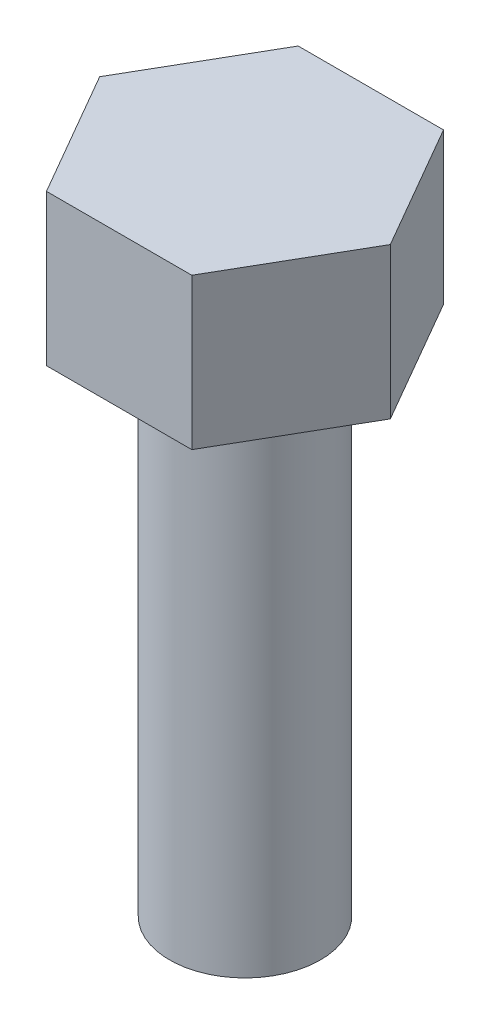
SolidWorks part; units mm, degrees
material "Plain Carbon Steel"
ref_plane "Front Plane" through (0, 0, 0) normal (0, 0, 1) x (1, 0, 0)
ref_plane "Top Plane" through (0, 0, 0) normal (0, 1, 0) x (1, 0, 0)
ref_plane "Right Plane" through (0, 0, 0) normal (1, 0, 0) x (0, 0, -1)
sketch "Hex Head Profile" plane through (0, 0, 0) normal (0, 1, 0) x (1, 0, 0)
  line L1 (2.8868, 0) -> (1.4434, 2.5)
  line L2 (1.4434, 2.5) -> (-1.4434, 2.5)
  line L3 (-1.4434, 2.5) -> (-2.8868, 0)
  line L4 (-2.8868, 0) -> (-1.4434, -2.5)
  line L5 (-1.4434, -2.5) -> (1.4434, -2.5)
  line L6 (1.4434, -2.5) -> (2.8868, 0)
  circle A0 centre (0, 0) radius 2.5 construction
  dimension "D1" = 5
extrude "Hex Head 5AF x 3" add sketch "Hex Head Profile" along normal blind 3
sketch "Shank Profile Ø3" plane through (0, 0, 0) normal (0, -1, 0) x (1, 0, 0)
  circle A0 centre (0, 0) radius 1.5
  dimension "D1" = 3
extrude "Shank Ø3 x 10" add sketch "Shank Profile Ø3" along normal blind 10 contours A0
